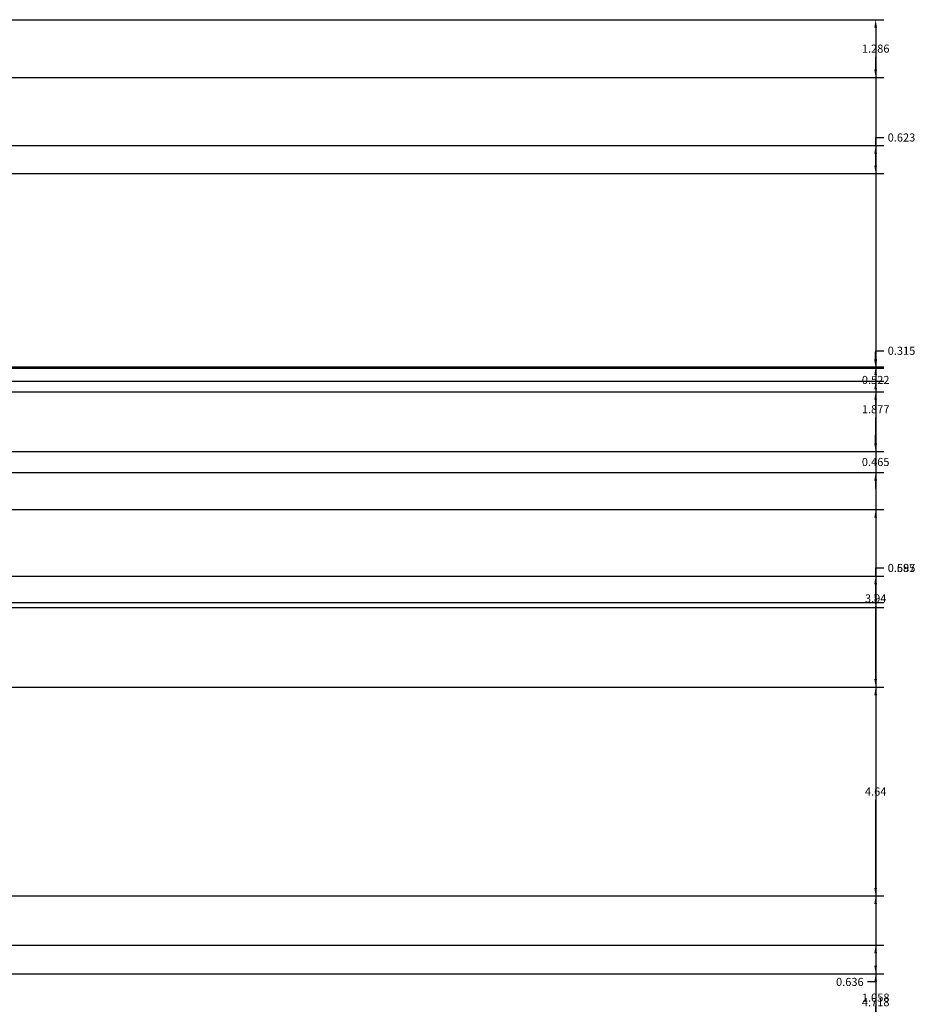
# Model space of a CAD drawing. Units: inches. Extents: x -10 to 130, y -32 to 34.
# Tile 22 of 22: x 110 to 130, y 5 to 27. Entities that reach past the tile are written whole.
import ezdxf

# ---------------------------------------------------------------- set-up
doc = ezdxf.new("R2010")
doc.units = ezdxf.units.IN
doc.header["$MEASUREMENT"] = 0
doc.layers.add('A-ANNO-DIMS', color=2, linetype='Continuous', lineweight=18)
doc.styles.get("Standard").update_dxf_attribs({"font": 'arial.ttf'})
doc.dimstyles.get("Standard").update_dxf_attribs({"dimtxt": 0.18, "dimasz": 0.18, "dimexe": 0.18, "dimexo": 0.0625, "dimgap": 0.09, "dimtad": 0, "dimtih": 1, "dimtoh": 1, "dimdec": 4, "dimzin": 0, "dimdsep": 46, "dimtxsty": 'Standard', "dimcen": 0.09, "dimadec": 0, "dimazin": 0, "dimtfac": 1, "dimtdec": 4, "dimtofl": 0, "dimtmove": 0, "dimatfit": 3, "dimfxl": 1, "dimtolj": 1, "dimtzin": 0, "dimarcsym": 0})

# ---------------------------------------------------------------- blocks, each defined once
blk = doc.blocks.new('*D2')
at = {"layer": 'A-ANNO-DIMS', "color": 0, "lineweight": -2, "transparency": 16777216}
for p, q in [((68.738, 27.199), (129.508, 27.199)), ((129.328, 27.019), (129.328, 3.074)), ((129.328, -21.234), (129.328, 2.71)), ((107.996, -21.414), (129.508, -21.414))]:
    blk.add_line(p, q, dxfattribs=at)
at = {"layer": 'A-ANNO-DIMS', "color": 0, "transparency": 16777216}
for points in [[(129.298, 27.019), (129.358, 27.019), (129.328, 27.199)], [(129.298, -21.234), (129.358, -21.234), (129.328, -21.414)]]:
    blk.add_solid(points, dxfattribs=at)
at = {"layer": 'Defpoints', "color": 0, "transparency": 16777216}
for p in [(68.676, 27.199), (129.328, 27.199), (107.933, -21.414)]:
    blk.add_point(p, dxfattribs=at)
at = {"layer": 'A-ANNO-DIMS', "color": 0, "transparency": 16777216, "insert": (129.328, 2.892), "char_height": 0.18, "attachment_point": 5}
blk.add_mtext('\\A1;48.61', dxfattribs=at)
blk = doc.blocks.new('*D79')
at = {"layer": 'A-ANNO-DIMS', "color": 0, "lineweight": -2, "transparency": 16777216}
for p, q in [((62.588, 7.736), (129.508, 7.736)), ((129.328, 7.556), (129.328, 5.559)), ((129.328, 3.198), (129.328, 5.195)), ((62.588, 3.018), (129.508, 3.018))]:
    blk.add_line(p, q, dxfattribs=at)
at = {"layer": 'A-ANNO-DIMS', "color": 0, "transparency": 16777216}
for points in [[(129.298, 7.556), (129.358, 7.556), (129.328, 7.736)], [(129.298, 3.198), (129.358, 3.198), (129.328, 3.018)]]:
    blk.add_solid(points, dxfattribs=at)
at = {"layer": 'Defpoints', "color": 0, "transparency": 16777216}
for p in [(62.526, 7.736), (129.328, 7.736), (62.526, 3.018)]:
    blk.add_point(p, dxfattribs=at)
at = {"layer": 'A-ANNO-DIMS', "color": 0, "transparency": 16777216, "insert": (129.328, 5.377), "char_height": 0.18, "attachment_point": 5}
blk.add_mtext('\\A1;4.718', dxfattribs=at)
blk = doc.blocks.new('*D80')
at = {"layer": 'A-ANNO-DIMS', "color": 0, "lineweight": -2, "transparency": 16777216}
for p, q in [((62.588, 12.373), (129.508, 12.373)), ((129.328, 12.193), (129.328, 10.237)), ((129.328, 7.916), (129.328, 9.873)), ((62.588, 7.736), (129.508, 7.736))]:
    blk.add_line(p, q, dxfattribs=at)
at = {"layer": 'A-ANNO-DIMS', "color": 0, "transparency": 16777216}
for points in [[(129.298, 12.193), (129.358, 12.193), (129.328, 12.373)], [(129.298, 7.916), (129.358, 7.916), (129.328, 7.736)]]:
    blk.add_solid(points, dxfattribs=at)
at = {"layer": 'Defpoints', "color": 0, "transparency": 16777216}
for p in [(62.526, 12.373), (129.328, 12.373), (62.526, 7.736)]:
    blk.add_point(p, dxfattribs=at)
at = {"layer": 'A-ANNO-DIMS', "color": 0, "transparency": 16777216, "insert": (129.328, 10.055), "char_height": 0.18, "attachment_point": 5}
blk.add_mtext('\\A1;4.64', dxfattribs=at)
blk = doc.blocks.new('*D81')
at = {"layer": 'A-ANNO-DIMS', "color": 0, "lineweight": -2, "transparency": 16777216}
for p, q in [((62.588, 16.317), (129.508, 16.317)), ((129.328, 16.137), (129.328, 14.527)), ((129.328, 12.553), (129.328, 14.163)), ((62.588, 12.373), (129.508, 12.373))]:
    blk.add_line(p, q, dxfattribs=at)
at = {"layer": 'A-ANNO-DIMS', "color": 0, "transparency": 16777216}
for points in [[(129.298, 16.137), (129.358, 16.137), (129.328, 16.317)], [(129.298, 12.553), (129.358, 12.553), (129.328, 12.373)]]:
    blk.add_solid(points, dxfattribs=at)
at = {"layer": 'Defpoints', "color": 0, "transparency": 16777216}
for p in [(62.526, 16.317), (129.328, 16.317), (62.526, 12.373)]:
    blk.add_point(p, dxfattribs=at)
at = {"layer": 'A-ANNO-DIMS', "color": 0, "transparency": 16777216, "insert": (129.328, 14.345), "char_height": 0.18, "attachment_point": 5}
blk.add_mtext('\\A1;3.94', dxfattribs=at)
blk = doc.blocks.new('*D82')
at = {"layer": 'A-ANNO-DIMS', "color": 0, "lineweight": -2, "transparency": 16777216}
for p, q in [((19.651, 19.485), (129.508, 19.485)), ((129.328, 19.305), (129.328, 18.728)), ((129.328, 17.787), (129.328, 18.364)), ((68.738, 17.607), (129.508, 17.607))]:
    blk.add_line(p, q, dxfattribs=at)
at = {"layer": 'A-ANNO-DIMS', "color": 0, "transparency": 16777216}
for points in [[(129.298, 19.305), (129.358, 19.305), (129.328, 19.485)], [(129.298, 17.787), (129.358, 17.787), (129.328, 17.607)]]:
    blk.add_solid(points, dxfattribs=at)
at = {"layer": 'Defpoints', "color": 0, "transparency": 16777216}
for p in [(19.588, 19.485), (68.676, 17.607), (129.328, 17.607)]:
    blk.add_point(p, dxfattribs=at)
at = {"layer": 'A-ANNO-DIMS', "color": 0, "transparency": 16777216, "insert": (129.328, 18.546), "char_height": 0.18, "attachment_point": 5}
blk.add_mtext('\\A1;1.877', dxfattribs=at)
blk = doc.blocks.new('*D85')
at = {"layer": 'A-ANNO-DIMS', "color": 0, "lineweight": -2, "transparency": 16777216}
for p, q in [((50.097, 27.199), (129.508, 27.199)), ((129.328, 27.019), (129.328, 26.738)), ((129.328, 26.093), (129.328, 26.374)), ((51.432, 25.913), (129.508, 25.913))]:
    blk.add_line(p, q, dxfattribs=at)
at = {"layer": 'A-ANNO-DIMS', "color": 0, "transparency": 16777216}
for points in [[(129.298, 27.019), (129.358, 27.019), (129.328, 27.199)], [(129.298, 26.093), (129.358, 26.093), (129.328, 25.913)]]:
    blk.add_solid(points, dxfattribs=at)
at = {"layer": 'Defpoints', "color": 0, "transparency": 16777216}
for p in [(50.035, 27.199), (129.328, 27.199), (51.37, 25.913)]:
    blk.add_point(p, dxfattribs=at)
at = {"layer": 'A-ANNO-DIMS', "color": 0, "transparency": 16777216, "insert": (129.328, 26.556), "char_height": 0.18, "attachment_point": 5}
blk.add_mtext('\\A1;1.286', dxfattribs=at)
blk = doc.blocks.new('*D108')
at = {"layer": 'A-ANNO-DIMS', "color": 0, "lineweight": -2, "transparency": 16777216}
for p, q in [((129.328, 14.841), (129.328, 15.021)), ((129.328, 15.021), (129.508, 15.021)), ((50.009, 14.841), (129.508, 14.841)), ((129.328, 14.436), (129.328, 14.661)), ((49.025, 14.256), (129.508, 14.256))]:
    blk.add_line(p, q, dxfattribs=at)
at = {"layer": 'A-ANNO-DIMS', "color": 0, "transparency": 16777216}
for points in [[(129.298, 14.661), (129.358, 14.661), (129.328, 14.841)], [(129.298, 14.436), (129.358, 14.436), (129.328, 14.256)]]:
    blk.add_solid(points, dxfattribs=at)
at = {"layer": 'Defpoints', "color": 0, "transparency": 16777216}
for p in [(49.946, 14.841), (129.328, 14.841), (48.963, 14.256)]:
    blk.add_point(p, dxfattribs=at)
at = {"layer": 'A-ANNO-DIMS', "color": 0, "transparency": 16777216, "insert": (129.902, 15.021), "char_height": 0.18, "attachment_point": 5}
blk.add_mtext('\\A1;0.585', dxfattribs=at)
blk = doc.blocks.new('*D138')
at = {"layer": 'A-ANNO-DIMS', "color": 0, "lineweight": -2, "transparency": 16777216}
for p, q in [((129.328, 14.841), (129.328, 15.021)), ((129.328, 15.021), (129.508, 15.021)), ((69.112, 14.841), (129.508, 14.841)), ((129.328, 14.324), (129.328, 14.661)), ((70.057, 14.144), (129.508, 14.144))]:
    blk.add_line(p, q, dxfattribs=at)
at = {"layer": 'A-ANNO-DIMS', "color": 0, "transparency": 16777216}
for points in [[(129.298, 14.661), (129.358, 14.661), (129.328, 14.841)], [(129.298, 14.324), (129.358, 14.324), (129.328, 14.144)]]:
    blk.add_solid(points, dxfattribs=at)
at = {"layer": 'Defpoints', "color": 0, "transparency": 16777216}
for p in [(69.05, 14.841), (129.328, 14.841), (69.995, 14.144)]:
    blk.add_point(p, dxfattribs=at)
at = {"layer": 'A-ANNO-DIMS', "color": 0, "transparency": 16777216, "insert": (129.901, 15.021), "char_height": 0.18, "attachment_point": 5}
blk.add_mtext('\\A1;0.697', dxfattribs=at)
blk = doc.blocks.new('*D139')
at = {"layer": 'A-ANNO-DIMS', "color": 0, "lineweight": -2, "transparency": 16777216}
for p, q in [((70.057, 6.643), (129.508, 6.643)), ((129.328, 6.463), (129.328, 6.187)), ((69.108, 6.007), (129.508, 6.007)), ((129.328, 6.007), (129.328, 5.827)), ((129.328, 5.827), (129.148, 5.827))]:
    blk.add_line(p, q, dxfattribs=at)
at = {"layer": 'A-ANNO-DIMS', "color": 0, "transparency": 16777216}
for points in [[(129.298, 6.463), (129.358, 6.463), (129.328, 6.643)], [(129.298, 6.187), (129.358, 6.187), (129.328, 6.007)]]:
    blk.add_solid(points, dxfattribs=at)
at = {"layer": 'Defpoints', "color": 0, "transparency": 16777216}
for p in [(69.995, 6.643), (69.045, 6.007), (129.328, 6.007)]:
    blk.add_point(p, dxfattribs=at)
at = {"layer": 'A-ANNO-DIMS', "color": 0, "transparency": 16777216, "insert": (128.754, 5.827), "char_height": 0.18, "attachment_point": 5}
blk.add_mtext('\\A1;0.636', dxfattribs=at)
blk = doc.blocks.new('*D142')
at = {"layer": 'A-ANNO-DIMS', "color": 0, "lineweight": -2, "transparency": 16777216}
for p, q in [((129.328, 19.665), (129.328, 19.845)), ((129.328, 19.845), (129.508, 19.845)), ((90.954, 19.485), (129.508, 19.485)), ((91.212, 19.17), (129.508, 19.17)), ((129.328, 18.99), (129.328, 18.81))]:
    blk.add_line(p, q, dxfattribs=at)
at = {"layer": 'A-ANNO-DIMS', "color": 0, "transparency": 16777216}
for points in [[(129.298, 19.665), (129.358, 19.665), (129.328, 19.485)], [(129.298, 18.99), (129.358, 18.99), (129.328, 19.17)]]:
    blk.add_solid(points, dxfattribs=at)
at = {"layer": 'Defpoints', "color": 0, "transparency": 16777216}
for p in [(90.892, 19.485), (129.328, 19.485), (91.15, 19.17)]:
    blk.add_point(p, dxfattribs=at)
at = {"layer": 'A-ANNO-DIMS', "color": 0, "transparency": 16777216, "insert": (129.902, 19.845), "char_height": 0.18, "attachment_point": 5}
blk.add_mtext('\\A1;0.315', dxfattribs=at)
blk = doc.blocks.new('*D145')
at = {"layer": 'A-ANNO-DIMS', "color": 0, "lineweight": -2, "transparency": 16777216}
for p, q in [((129.328, 24.402), (129.328, 24.582)), ((129.328, 24.582), (129.508, 24.582)), ((82.677, 24.402), (129.508, 24.402)), ((129.328, 23.959), (129.328, 24.222)), ((83.241, 23.779), (129.508, 23.779))]:
    blk.add_line(p, q, dxfattribs=at)
at = {"layer": 'A-ANNO-DIMS', "color": 0, "transparency": 16777216}
for points in [[(129.298, 24.222), (129.358, 24.222), (129.328, 24.402)], [(129.298, 23.959), (129.358, 23.959), (129.328, 23.779)]]:
    blk.add_solid(points, dxfattribs=at)
at = {"layer": 'Defpoints', "color": 0, "transparency": 16777216}
for p in [(82.614, 24.402), (129.328, 24.402), (83.179, 23.779)]:
    blk.add_point(p, dxfattribs=at)
at = {"layer": 'A-ANNO-DIMS', "color": 0, "transparency": 16777216, "insert": (129.901, 24.582), "char_height": 0.18, "attachment_point": 5}
blk.add_mtext('\\A1;0.623', dxfattribs=at)
blk = doc.blocks.new('*D148')
at = {"layer": 'A-ANNO-DIMS', "color": 0, "lineweight": -2, "transparency": 16777216}
for p, q in [((129.327673, 19.637521), (129.327673, 19.817521)), ((79.689531, 19.457521), (129.507673, 19.457521)), ((80.07533, 18.935883), (129.507673, 18.935883)), ((129.327673, 18.755883), (129.327673, 18.575883))]:
    blk.add_line(p, q, dxfattribs=at)
at = {"layer": 'A-ANNO-DIMS', "color": 0, "transparency": 16777216}
for points in [[(129.297673, 19.637521), (129.357673, 19.637521), (129.327673, 19.457521)], [(129.297673, 18.755883), (129.357673, 18.755883), (129.327673, 18.935883)]]:
    blk.add_solid(points, dxfattribs=at)
at = {"layer": 'Defpoints', "color": 0, "transparency": 16777216}
for p in [(79.627031, 19.457521), (129.327673, 19.457521), (80.01283, 18.935883)]:
    blk.add_point(p, dxfattribs=at)
at = {"layer": 'A-ANNO-DIMS', "color": 0, "transparency": 16777216, "insert": (129.327673, 19.196702), "char_height": 0.18, "attachment_point": 5}
blk.add_mtext('\\A1;0.522', dxfattribs=at)
blk = doc.blocks.new('*D150')
at = {"layer": 'A-ANNO-DIMS', "color": 0, "lineweight": -2, "transparency": 16777216}
for p, q in [((129.327673, 17.787359), (129.327673, 17.967359)), ((74.432221, 17.607359), (129.507673, 17.607359)), ((73.944831, 17.142679), (129.507673, 17.142679)), ((129.327673, 16.962679), (129.327673, 16.782679))]:
    blk.add_line(p, q, dxfattribs=at)
at = {"layer": 'A-ANNO-DIMS', "color": 0, "transparency": 16777216}
for points in [[(129.297673, 17.787359), (129.357673, 17.787359), (129.327673, 17.607359)], [(129.297673, 16.962679), (129.357673, 16.962679), (129.327673, 17.142679)]]:
    blk.add_solid(points, dxfattribs=at)
at = {"layer": 'Defpoints', "color": 0, "transparency": 16777216}
for p in [(74.369721, 17.607359), (129.327673, 17.607359), (73.882331, 17.142679)]:
    blk.add_point(p, dxfattribs=at)
at = {"layer": 'A-ANNO-DIMS', "color": 0, "transparency": 16777216, "insert": (129.327673, 17.375019), "char_height": 0.18, "attachment_point": 5}
blk.add_mtext('\\A1;0.465', dxfattribs=at)
blk = doc.blocks.new('*D154')
at = {"layer": 'A-ANNO-DIMS', "color": 0, "lineweight": -2, "transparency": 16777216}
for p, q in [((81.468, 6.007), (129.508, 6.007)), ((129.328, 5.827), (129.328, 3.941)), ((129.328, 1.691), (129.328, 3.577)), ((81.468, 1.511), (129.508, 1.511))]:
    blk.add_line(p, q, dxfattribs=at)
at = {"layer": 'A-ANNO-DIMS', "color": 0, "transparency": 16777216}
for points in [[(129.298, 5.827), (129.358, 5.827), (129.328, 6.007)], [(129.298, 1.691), (129.358, 1.691), (129.328, 1.511)]]:
    blk.add_solid(points, dxfattribs=at)
at = {"layer": 'Defpoints', "color": 0, "transparency": 16777216}
for p in [(81.405, 6.007), (129.328, 6.007), (81.405, 1.511)]:
    blk.add_point(p, dxfattribs=at)
at = {"layer": 'A-ANNO-DIMS', "color": 0, "transparency": 16777216, "insert": (129.328, 3.759), "char_height": 0.18, "attachment_point": 5}
blk.add_mtext('\\A1;4.497', dxfattribs=at)
blk = doc.blocks.new('*D161')
at = {"layer": 'A-ANNO-DIMS', "color": 0, "lineweight": -2, "transparency": 16777216}
for p, q in [((94.793, 6.007), (129.508, 6.007)), ((129.328, 5.827), (129.328, 5.064)), ((129.328, 3.936), (129.328, 4.7)), ((94.793, 3.756), (129.508, 3.756))]:
    blk.add_line(p, q, dxfattribs=at)
at = {"layer": 'A-ANNO-DIMS', "color": 0, "transparency": 16777216}
for points in [[(129.298, 5.827), (129.358, 5.827), (129.328, 6.007)], [(129.298, 3.936), (129.358, 3.936), (129.328, 3.756)]]:
    blk.add_solid(points, dxfattribs=at)
at = {"layer": 'Defpoints', "color": 0, "transparency": 16777216}
for p in [(94.73, 6.007), (94.73, 3.756), (129.328, 3.756)]:
    blk.add_point(p, dxfattribs=at)
at = {"layer": 'A-ANNO-DIMS', "color": 0, "transparency": 16777216, "insert": (129.328, 4.882), "char_height": 0.18, "attachment_point": 5}
blk.add_mtext('\\A1;2.252', dxfattribs=at)
blk = doc.blocks.new('*D165')
at = {"layer": 'A-ANNO-DIMS', "color": 0, "lineweight": -2, "transparency": 16777216}
for p, q in [((94.793, 6.007), (129.508, 6.007)), ((129.328, 5.827), (129.328, 5.66)), ((129.328, 5.13), (129.328, 5.297)), ((96.123, 4.95), (129.508, 4.95))]:
    blk.add_line(p, q, dxfattribs=at)
at = {"layer": 'A-ANNO-DIMS', "color": 0, "transparency": 16777216}
for points in [[(129.298, 5.827), (129.358, 5.827), (129.328, 6.007)], [(129.298, 5.13), (129.358, 5.13), (129.328, 4.95)]]:
    blk.add_solid(points, dxfattribs=at)
at = {"layer": 'Defpoints', "color": 0, "transparency": 16777216}
for p in [(94.73, 6.007), (129.328, 6.007), (96.061, 4.95)]:
    blk.add_point(p, dxfattribs=at)
at = {"layer": 'A-ANNO-DIMS', "color": 0, "transparency": 16777216, "insert": (129.328, 5.478), "char_height": 0.18, "attachment_point": 5}
blk.add_mtext('\\A1;1.058', dxfattribs=at)

msp = doc.modelspace()

# ---------------------------------------------------------------- dimensions: what is measured, and where the dimension line sits
at = {"layer": 'A-ANNO-DIMS'}
for base, p1, p2, override, picture, middle in [((129.3277, 27.1987), (51.3699, 25.9127), (50.0347, 27.1987), {"dimdec": 3, "dimlfac": 1, "dimrnd": 0, "dimzin": 0, "dimdsep": 46, "dimlunit": 2}, '*D85', (129.3277, 26.5557)), ((129.3277, 27.1987), (107.9333, -21.4145), (68.6759, 27.1987), {"dimdec": 2, "dimlfac": 1, "dimrnd": 0, "dimzin": 0, "dimdsep": 46, "dimlunit": 2}, '*D2', (129.3277, 2.8921)), ((129.3277, 24.4019), (83.1789, 23.7785), (82.6141, 24.4019), {"dimdec": 3, "dimlfac": 1, "dimrnd": 0, "dimzin": 0, "dimdsep": 46, "dimlunit": 2}, '*D145', (129.9014, 24.5819)), ((129.3277, 19.4845), (91.1497, 19.1697), (90.8917, 19.4845), {"dimdec": 3, "dimlfac": 1, "dimrnd": 0, "dimzin": 0, "dimdsep": 46, "dimlunit": 2}, '*D142', (129.9021, 19.8445)), ((129.3277, 19.4575), (80.0128, 18.9359), (79.627, 19.4575), {"dimdec": 3, "dimlfac": 1, "dimrnd": 0, "dimzin": 0, "dimdsep": 46, "dimlunit": 2}, '*D148', (129.3277, 19.1967)), ((129.3277, 17.6074), (19.5881, 19.4845), (68.6759, 17.6074), {"dimdec": 3, "dimlfac": 1, "dimrnd": 0, "dimzin": 0, "dimdsep": 46, "dimlunit": 2}, '*D82', (129.3277, 18.5459)), ((129.3277, 17.6074), (73.8823, 17.1427), (74.3697, 17.6074), {"dimdec": 3, "dimlfac": 1, "dimrnd": 0, "dimzin": 0, "dimdsep": 46, "dimlunit": 2}, '*D150', (129.3277, 17.375)), ((129.3277, 16.3174), (62.5256, 12.3729), (62.5256, 16.3174), {"dimdec": 2, "dimlfac": 1, "dimrnd": 0, "dimzin": 0, "dimdsep": 46, "dimlunit": 2}, '*D81', (129.3277, 14.3452)), ((129.3277, 14.8409), (48.963, 14.2556), (49.9462, 14.8409), {"dimdec": 3, "dimlfac": 1, "dimrnd": 0, "dimzin": 0, "dimdsep": 46, "dimlunit": 2}, '*D108', (129.9021, 15.0209)), ((129.3277, 14.8409), (69.9946, 14.144), (69.0498, 14.8409), {"dimdec": 3, "dimlfac": 1, "dimrnd": 0, "dimzin": 0, "dimdsep": 46, "dimlunit": 2}, '*D138', (129.9014, 15.0209)), ((129.3277, 12.3729), (62.5256, 7.7364), (62.5256, 12.3729), {"dimdec": 2, "dimlfac": 1, "dimrnd": 0, "dimzin": 0, "dimdsep": 46, "dimlunit": 2}, '*D80', (129.3277, 10.0547)), ((129.3277, 7.7364), (62.5256, 3.0181), (62.5256, 7.7364), {"dimdec": 3, "dimlfac": 1, "dimrnd": 0, "dimzin": 0, "dimdsep": 46, "dimlunit": 2}, '*D79', (129.3277, 5.3773)), ((129.3277, 6.0074), (69.9946, 6.6433), (69.0452, 6.0074), {"dimdec": 3, "dimlfac": 1, "dimrnd": 0, "dimzin": 0, "dimdsep": 46, "dimlunit": 2}, '*D139', (128.754, 5.8274)), ((129.3277, 6.0074), (81.4053, 1.5107), (81.4053, 6.0074), {"dimdec": 3, "dimlfac": 1, "dimrnd": 0, "dimzin": 0, "dimdsep": 46, "dimlunit": 2}, '*D154', (129.3277, 3.7591)), ((129.3277, 3.7558), (94.7302, 6.0074), (94.7302, 3.7558), {"dimdec": 3, "dimlfac": 1, "dimrnd": 0, "dimzin": 0, "dimdsep": 46, "dimlunit": 2}, '*D161', (129.3277, 4.8816)), ((129.3277, 6.0074), (96.0606, 4.9495), (94.7302, 6.0074), {"dimdec": 3, "dimlfac": 1, "dimrnd": 0, "dimzin": 0, "dimdsep": 46, "dimlunit": 2}, '*D165', (129.3277, 5.4785))]:
    dim = msp.add_linear_dim(base=base, p1=p1, p2=p2, angle=90, dimstyle='Standard', override=override, dxfattribs=at)
    dim.commit()
    dim.dimension.update_dxf_attribs({"geometry": picture, "text_midpoint": middle})

doc.saveas('drawing.dxf')
